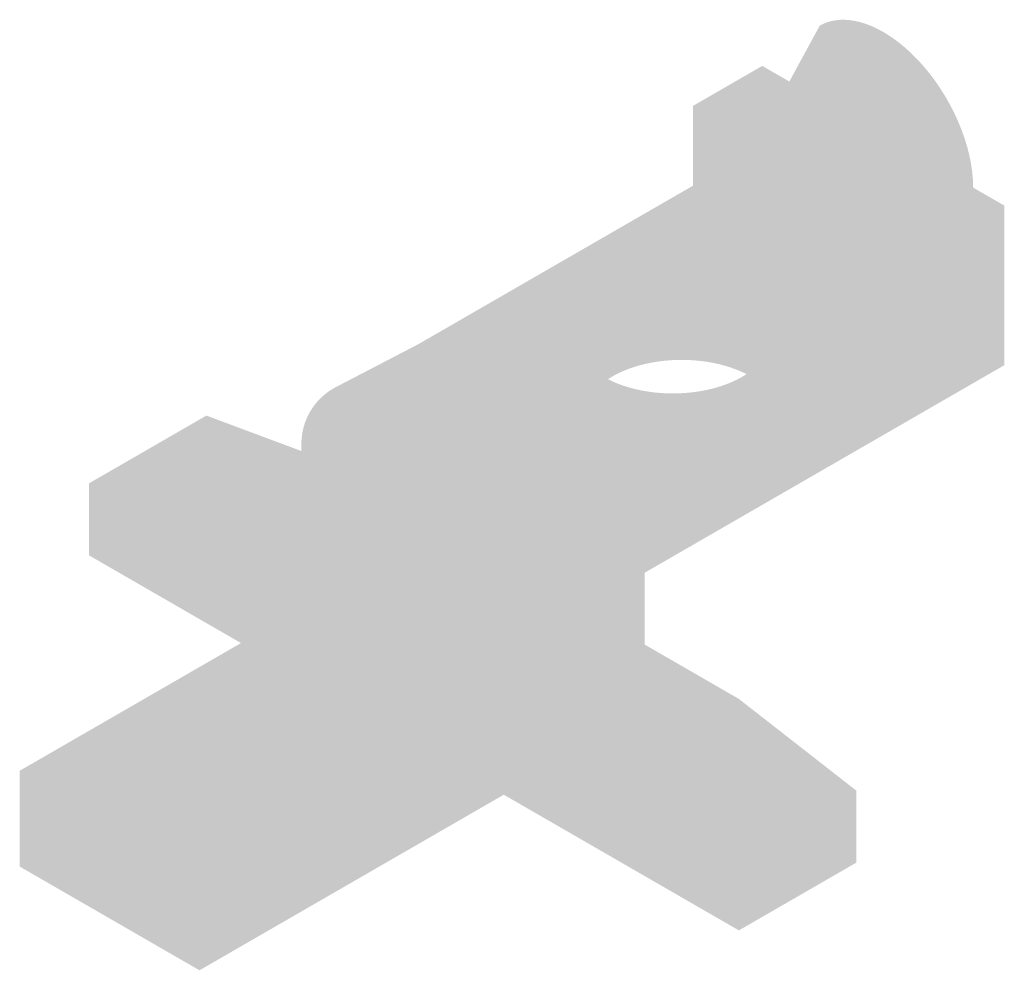
# Model space of a CAD drawing. Units: inches. Extents: x 1177 to 33026, y 779 to 22841.
# Tile 1 of 2: x 1177 to 1300, y 779 to 898. Entities that reach past the tile are written whole.
import ezdxf

# ---------------------------------------------------------------- set-up
doc = ezdxf.new("R2010")
doc.units = ezdxf.units.IN
doc.header["$MEASUREMENT"] = 0
doc.layers.add('M-HATC', color=18, linetype='Continuous', lineweight=18)

msp = doc.modelspace()

# ---------------------------------------------------------------- hatches: boundary and pattern name
at = {"layer": 'M-HATC'}
h = msp.add_hatch(color=256, dxfattribs=at)
h.dxf.hatch_style = 1
h.set_gradient(color1=(99, 100, 102), tint=1, name='INVCYLINDER')
edge = h.paths.add_edge_path()
edge.add_line((1291.451790575787, 859.9577290049253), (1291.451790575787, 869.9577290049255))
edge.add_line((1291.451790575787, 869.9577290049255), (1283.224549239835, 874.7077290049253))
edge.add_ellipse((1276.29634600956, 878.7077290049253), major_axis=(4.898979485566418, -8.485281374238538), ratio=0.5773502691896235, start_angle=29.99999999999987, end_angle=179.999999999998)
edge.add_ellipse((1276.29634600956, 878.7077290049253), major_axis=(4.898979485566418, -8.485281374238538), ratio=0.5773502691896235, start_angle=179.999999999998, end_angle=209.9999999999999)
edge.add_line((1269.368142779284, 882.7077290049253), (1261.140901443332, 887.4577290049255))
edge.add_line((1261.140901443332, 887.4577290049255), (1261.140901443332, 877.4577290049255))
edge.add_line((1261.140901443332, 877.4577290049255), (1226.738732631339, 857.5956275806143))
edge.add_line((1226.738732631339, 857.5956275806143), (1216.390617514184, 852.2089768709296))
edge.add_arc((1220.084478519672, 845.1128236262382), 8, 117.4989673014574, 180)
edge.add_line((1212.084478519672, 845.1128236262382), (1212.084478519672, 827.7805179733663))
edge.add_line((1212.084478519672, 827.7805179733663), (1214.913523706214, 826.1471679733663))
edge.add_line((1214.913523706214, 826.1471679733663), (1237.430184204609, 813.1471679733662))
edge.add_line((1237.430184204609, 813.1471679733662), (1240.361335680709, 811.4548668796043))
edge.add_line((1240.361335680709, 811.4548668796043), (1240.361335680709, 825.841838964715))
edge.add_arc((1248.361335680709, 825.8418389647147), 7.999999999999974, 120.0000000000002, 179.9999999999992, ccw=False)
edge.add_line((1244.361335680709, 832.7700421949902), (1255.078723616841, 838.9577290049256))
edge.add_line((1255.078723616841, 838.9577290049256), (1291.451790575787, 859.9577290049253))
edge = h.paths.add_edge_path(flags=16)
edge.add_ellipse((1258.602537066825, 858.4922036488476), major_axis=(-12.24744871391589, 0), ratio=0.5773502691896212, start_angle=153.2412704775436, end_angle=393.0442202934223, ccw=False)
edge.add_ellipse((1258.602537066825, 858.4922036488476), major_axis=(-12.24744871391589, 0), ratio=0.5773502691896212, start_angle=33.04422029342231, end_angle=153.2412704775436, ccw=False)
edge = h.paths.add_edge_path(flags=0)
edge.add_ellipse((1258.602537066825, 858.4922036488476), major_axis=(-12.24744871391589, 0), ratio=0.5773502691896212, start_angle=153.2412704775436, end_angle=393.0442202934223)
edge.add_ellipse((1259.697328146386, 848.5523126790175), major_axis=(-12.24744871391589, 0), ratio=0.5773502691896212, start_angle=213.0442202929725, end_angle=333.2412704775611, ccw=False)
edge = h.paths.add_edge_path()
edge.add_line((1273.193722100556, 890.4990297539823), (1269.801155481177, 892.4577290049251))
edge.add_line((1269.801155481177, 892.4577290049251), (1261.140901443332, 887.4577290049255))
edge.add_line((1261.140901443332, 887.4577290049255), (1269.368142779284, 882.7077290049253))
edge.add_ellipse((1276.29634600956, 878.7077290049253), major_axis=(4.898979485566418, -8.485281374238538), ratio=0.5773502691896235, start_angle=179.9999999999981, end_angle=209.9999999999999, ccw=False)
edge.add_line((1271.397366523993, 887.1930103791638), (1273.193722100556, 890.4990297539823))
edge = h.paths.add_edge_path()
edge.add_ellipse((1284.956600047404, 883.7077290049252), major_axis=(7.960841664045289, -13.7885822331377), ratio=0.5773502691896263, start_angle=390.0000000000008, end_angle=540)
edge.add_line((1276.995758383359, 897.4963112380631), (1271.397366523993, 887.1930103791639))
edge.add_ellipse((1276.29634600956, 878.7077290049253), major_axis=(4.898979485566418, -8.485281374238538), ratio=0.5773502691896235, start_angle=29.999999999999886, end_angle=179.9999999999981, ccw=False)
edge.add_line((1283.224549239835, 874.7077290049253), (1296.214930296602, 877.2077290049255))
h.paths.add_polyline_path([(1300.112044613632, 874.9577290049255), (1296.214930296602, 877.2077290049255), (1283.224549239835, 874.7077290049253), (1291.451790575787, 869.9577290049255)])
h.paths.add_polyline_path([(1255.078723616841, 828.9577290049255), (1291.451790575787, 849.9577290049255), (1300.112044613632, 854.9577290049255), (1300.112044613632, 874.9577290049255), (1291.451790575787, 869.9577290049255), (1291.451790575787, 859.9577290049253), (1255.078723616841, 838.9577290049256), (1244.361335680709, 832.7700421949902, 0.2679491924311165), (1240.361335680709, 825.841838964715), (1240.361335680709, 811.4548668796047), (1255.078723616841, 819.9577290049255)])
h.paths.add_polyline_path([(1212.084478519672, 844.2040003362018), (1200.191048551013, 848.6471429793736), (1185.468659977543, 840.1471679733663), (1200.19109184188, 834.6471679733658), (1212.084478519672, 827.7805179733663)])
h.paths.add_polyline_path([(1200.19109184188, 834.6471679733658), (1185.468659977543, 840.1471679733663), (1185.468659977543, 831.1471679733664), (1204.521218860801, 820.1471679733662), (1214.913523706214, 826.1471679733663)])
h.paths.add_polyline_path([(1252.152616068947, 804.6471679733648), (1237.430184204609, 813.1471679733662), (1237.430184204609, 801.1471679733663), (1266.87504793328, 784.1471679733663), (1266.87504793328, 793.1471679733663)])
h.paths.add_polyline_path([(1266.87504793328, 813.1471179853809), (1255.078723616841, 819.9577290049255), (1240.361335680709, 811.4548668796047), (1252.152616068947, 804.6471679733648), (1266.87504793328, 793.1471679733663), (1281.597479797616, 801.6471179853809)])
edge = h.paths.add_edge_path()
edge.add_ellipse((1209.717371283507, 810.1471679733661), major_axis=(-11.02270384252403, 0), ratio=0.5773502691896241, start_angle=150.0000000000011, end_angle=154.9876795157223)
edge.add_ellipse((1209.717371283507, 802.1471679733659), major_axis=(-11.02270384252403, 0), ratio=0.577350269189624, start_angle=205.0123204842778, end_angle=330.0000000000018)
edge.add_line((1201.923142649449, 806.6471679733663), (1180.272507554837, 794.147167973366))
edge.add_line((1180.272507554837, 794.147167973366), (1195.860964822956, 785.1471679733662))
edge.add_line((1195.860964822956, 785.1471679733662), (1195.860964822956, 793.1471679733663))
edge.add_line((1195.860964822956, 793.1471679733663), (1217.511599917567, 805.6471679733663))
edge = h.paths.add_edge_path(flags=16)
edge.add_ellipse((1209.717371283507, 802.1471679733659), major_axis=(-11.02270384252403, 0), ratio=0.577350269189624, start_angle=205.0123204842779, end_angle=330.0000000000018, ccw=False)
edge.add_ellipse((1209.717371283507, 810.1471679733661), major_axis=(-11.02270384252403, 0), ratio=0.5773502691896241, start_angle=154.9876795157223, end_angle=330.0000000000018)
edge.add_line((1201.923142649448, 814.6471679733664), (1180.272507554836, 802.1471679733659))
edge.add_line((1180.272507554836, 802.1471679733659), (1180.272507554836, 794.1471679733656))
edge.add_line((1180.272507554836, 794.1471679733656), (1201.92314264945, 806.6471679733668))
h.paths.add_polyline_path([(1237.430184204609, 813.1471679733662), (1214.913523706214, 826.1471679733663), (1204.521218860801, 820.1471679733662), (1176.808405939699, 804.1471679733662), (1180.272507554836, 802.1471679733659), (1180.272507554836, 794.1471679733663), (1195.860964822956, 785.1471679733662), (1195.860964822956, 793.1471679733661), (1199.325066438094, 791.1471679733663)])
h.paths.add_polyline_path([(1237.430184204609, 801.1471679733663), (1237.430184204609, 813.1471679733662), (1199.325066438094, 791.1471679733663), (1199.325066438094, 779.1471679733663)])
h.paths.add_polyline_path([(1199.325066438094, 791.1471679733663), (1195.860964822956, 793.1471679733661), (1195.860964822956, 785.1471679733662), (1180.272507554836, 794.1471679733663), (1180.272507554836, 802.1471679733659), (1176.808405939699, 804.1471679733662), (1176.808405939699, 792.1471679733663), (1199.325066438094, 779.1471679733663)])
h = msp.add_hatch(color=256, dxfattribs=at)
h.dxf.hatch_style = 1
h.set_gradient(color1=(99, 100, 102), name='INVCYLINDER')
h.paths.add_polyline_path([(1281.597479797616, 792.6471679733663), (1281.597479797616, 801.6471179853809), (1266.87504793328, 793.1471679733663), (1266.87504793328, 784.1471679733663)])
edge = h.paths.add_edge_path()
edge.add_ellipse((1209.717371283507, 810.1471679733661), major_axis=(-11.02270384252403, 0), ratio=0.5773502691896241, start_angle=150.0000000000011, end_angle=154.9876795157223)
edge.add_ellipse((1209.717371283507, 802.1471679733659), major_axis=(-11.02270384252403, 0), ratio=0.577350269189624, start_angle=205.0123204842778, end_angle=330.0000000000018)
edge.add_line((1201.923142649448, 806.6471679733663), (1180.272507554837, 794.147167973366))
edge.add_line((1180.272507554837, 794.147167973366), (1195.860964822956, 785.1471679733662))
edge.add_line((1195.860964822956, 785.1471679733662), (1195.860964822956, 793.1471679733663))
edge.add_line((1195.860964822956, 793.1471679733663), (1217.511599917567, 805.6471679733663))
h.paths.add_polyline_path([(1226.171853955412, 819.6471679733663), (1214.913523706214, 826.1471679733663), (1176.808405939699, 804.1471679733662), (1180.272507554836, 802.1471679733659), (1180.272507554836, 794.1471679733663), (1195.860964822956, 785.1471679733662), (1195.860964822956, 793.1471679733661), (1199.325066438094, 791.1471679733663), (1237.430184204609, 813.1471679733662)])
edge = h.paths.add_edge_path()
edge.add_ellipse((1258.602537066825, 858.4922036488476), major_axis=(-12.24744871391589, 0), ratio=0.5773502691896212, start_angle=153.2412704775436, end_angle=393.0442202934223)
edge.add_ellipse((1259.697328146386, 848.5523126790175), major_axis=(-12.24744871391589, 0), ratio=0.5773502691896212, start_angle=213.0442202929725, end_angle=333.2412704775611, ccw=False)
h = msp.add_hatch(color=256, dxfattribs=at)
h.dxf.hatch_style = 1
h.set_gradient(color1=(99, 100, 102), name='INVCYLINDER')
edge = h.paths.add_edge_path()
edge.add_ellipse((1209.717371283507, 810.1471679733661), major_axis=(-11.02270384252403, 0), ratio=0.5773502691896241, start_angle=150.0000000000011, end_angle=154.9876795157223)
edge.add_ellipse((1209.717371283507, 802.1471679733659), major_axis=(-11.02270384252403, 0), ratio=0.577350269189624, start_angle=205.0123204842778, end_angle=330.0000000000018)
edge.add_line((1201.923142649449, 806.6471679733663), (1180.272507554837, 794.147167973366))
edge.add_line((1180.272507554837, 794.147167973366), (1195.860964822956, 785.1471679733662))
edge.add_line((1195.860964822956, 785.1471679733662), (1195.860964822956, 793.1471679733663))
edge.add_line((1195.860964822956, 793.1471679733663), (1217.511599917567, 805.6471679733663))

doc.saveas('drawing.dxf')
